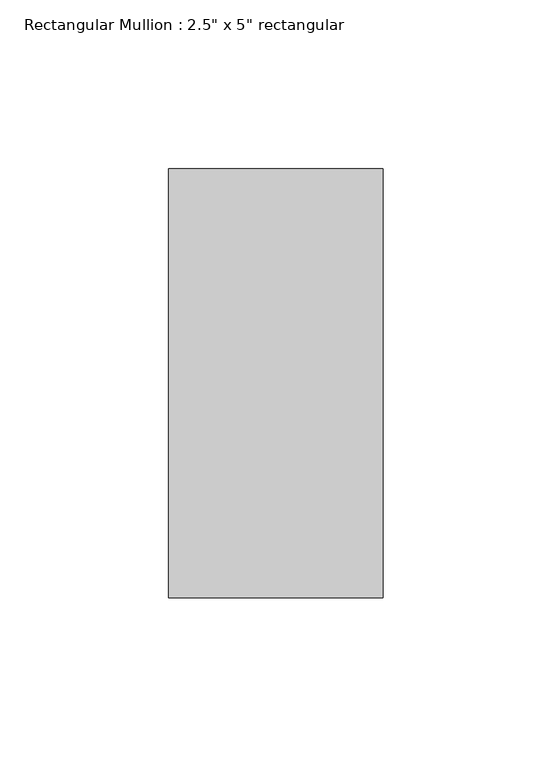
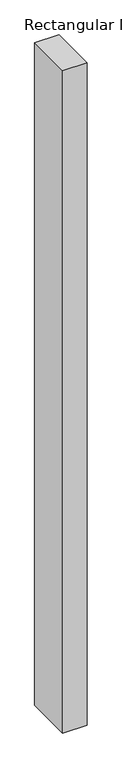
"""IFC4 building model written with IfcOpenShell, lengths in millimetres: member geometry."""

from ifc_helpers import new_model, si_unit, frame, origin, place, context, project, spatial, polyline, outline, extrude, source, transform, mapped, element, save


def member_d60e8053(model_context):
    return source(origin(), model_context, "Body", "SweptSolid", [
        extrude(outline(polyline([(31.75, 63.5), (31.75, -63.5), (-31.75, -63.5), (-31.75, 63.5), (31.75, 63.5)])), frame((0.0, 0.0, -1828.8), z_axis=(0.0, 0.0, 1.0), x_axis=(1.0, 0.0, 0.0)), (0.0, 0.0, 1.0), 1828.8),
    ])


if __name__ == "__main__":
    model = new_model("IFC4")
    model_context = context("Model", 3, world=origin())
    ifc_project = project(units=[si_unit("LENGTHUNIT", "METRE", prefix="MILLI")], contexts=[model_context])
    site = spatial("IfcSite", under=ifc_project)
    building = spatial("IfcBuilding", under=site)
    placement = place(None, origin())
    member_shape = member_d60e8053(model_context)
    element("IfcMember", 1, ObjectType="Rectangular Mullion : 2.5\" x 5\" rectangular", at=placement, inside=building, context=model_context, shape_type="MappedRepresentation", body=[
        mapped(member_shape, transform((0.0, 0.0, 0.0), x_axis=(1.0, 0.0, 0.0), y_axis=(0.0, 1.0, 0.0), z_axis=(0.0, 0.0, 1.0))),
    ])
    save(model, "model.ifc")

# Revit data of these elements
# Type "Rectangular Mullion : 2.5\" x 5\" rectangular"
#   built-in parameter 1007304 = 0.416667 (stored number, unit not read)
#   built-in parameter 1007301 = 0.104167 (stored number, unit not read)
#   built-in parameter 1007300 = 0.104167 (stored number, unit not read)
